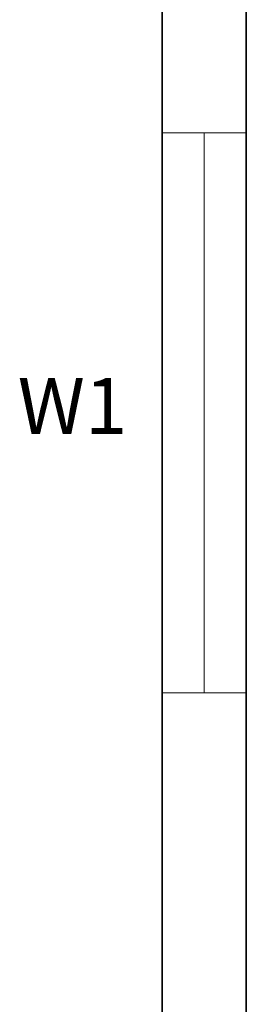
# Model space of a CAD drawing. Units: inches. Extents: x -36302355 to 648, y -221479757 to 75.
# Tile 11 of 37: x 259 to 283, y -531 to -425. Entities that reach past the tile are written whole.
import ezdxf

# ---------------------------------------------------------------- set-up
doc = ezdxf.new("R2010")
doc.units = ezdxf.units.IN
doc.header["$MEASUREMENT"] = 0
for name, color, linetype, lineweight in [('A-ANNO-IDEN', 7, 'Continuous', 18), ('A-GLAZ', 142, 'Continuous', 18), ('A-WALL', 7, 'Continuous', 35)]:
    doc.layers.add(name, color=color, linetype=linetype, lineweight=lineweight)
doc.styles.get("Standard").update_dxf_attribs({"font": 'arial.ttf'})

# ---------------------------------------------------------------- blocks, each defined once
blk = doc.blocks.new('WIN-60')
for p, q in [((60, 9), (0, 9)), ((0, 9), (0, 0)), ((60, 0), (60, 9)), ((0, 4.5), (60, 4.5)), ((0, 0), (60, 0))]:
    blk.add_line(p, q)

msp = doc.modelspace()

# ---------------------------------------------------------------- linework, layer by layer
at = {"layer": 'A-WALL'}
for p, q in [((274.2, -309.52), (274.2, -580.02)), ((283.2, -374.52), (283.2, -580.02))]:
    msp.add_line(p, q, dxfattribs=at)

# ---------------------------------------------------------------- block references
at = {"layer": 'A-GLAZ', "extrusion": (0, 0, -1), "zscale": -1, "rotation": 90}
msp.add_blockref('WIN-60', (-274.2, -497.29), dxfattribs=at)

# ---------------------------------------------------------------- texts
at = {"layer": 'A-ANNO-IDEN', "insert": (258.75, -463.55), "char_height": 6, "attachment_point": 1}
msp.add_mtext_dynamic_manual_height_columns('W1', width=0.8021, gutter_width=1, heights=[0], dxfattribs=at)

doc.saveas('drawing.dxf')
